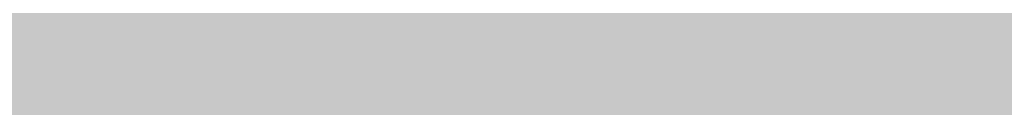
# Model space of a CAD drawing. Units: inches. Extents: x 2091 to 2899, y 967 to 2217.
# Tile 230 of 256: x 2203.4104 to 2203.7172, y 1152.274 to 1152.3009. Entities that reach past the tile are written whole.
import ezdxf

# ---------------------------------------------------------------- set-up
doc = ezdxf.new("R2010")
doc.units = ezdxf.units.IN
doc.layers.add('A-WALL-PATT', color=141, linetype='Continuous', lineweight=13, true_color=0xadddf7)

msp = doc.modelspace()

# ---------------------------------------------------------------- hatches: boundary and pattern name
at = {"layer": 'A-WALL-PATT'}
h = msp.add_hatch(color=256, dxfattribs=at)
h.dxf.hatch_style = 1
h.paths.add_polyline_path([(2803.1436, 2050.91906), (2203.1436, 2050.91906), (2203.1436, 1090.91906), (2803.1436, 1090.91906)])
h.paths.add_polyline_path([(2635.79885, 1147.54046), (2674.52405, 1147.54046, 0.376086), (2678.52967, 1152.8802), (2678.52967, 1159.55647, 0.333335), (2674.52432, 1163.56185), (2674.52432, 1163.56185), (2674.52432, 1192.93439), (2635.80597, 1192.93439), (2597.08762, 1192.93439), (2597.08762, 1163.56185, 0.333335), (2593.08228, 1159.55647), (2593.08228, 1152.8802, 0.376086), (2597.08789, 1147.54046)], flags=0)
h.paths.add_polyline_path([(2436.01043, 1278.24078, 0.000483), (2435.95264, 1278.21503, -0.001328), (2435.93563, 1278.11169, -0.001711), (2436.11644, 1278.04076, 0.002185)], flags=0)
h.paths.add_polyline_path([(2794.1436, 1143.41906), (2794.1436, 1347.41906), (2543.37017, 1347.41906), (2543.37017, 1351.91906), (2794.1436, 1351.91906), (2794.1436, 1392.71355), (2793.9474, 1392.71355), (2793.9474, 1473.5369), (2794.1436, 1473.5369), (2794.1436, 1531.91906), (2650.1436, 1531.91906), (2650.1436, 1536.41906), (2794.1436, 1536.41906), (2794.1436, 1692.41906), (2609.37561, 1692.41906), (2609.37561, 1644.41906), (2604.87561, 1644.41906), (2604.87561, 1744.91906), (2609.37561, 1744.91906), (2609.37561, 1696.91906), (2794.1436, 1696.91906), (2794.1436, 1780.91906), (2609.6436, 1780.91906), (2493.87561, 1780.91906), (2493.87561, 1785.41906), (2609.6436, 1785.41906), (2794.1436, 1785.41906), (2794.1436, 1847.93882), (2793.95122, 1847.93882), (2793.95122, 1928.76217), (2794.1436, 1928.76217), (2794.1436, 1941.41906), (2614.1436, 1941.41906), (2614.1436, 1821.41906), (2609.6436, 1821.41906), (2609.6436, 1941.41906), (2392.1436, 1941.41906), (2392.1436, 1819.91906), (2387.6436, 1819.91906), (2387.6436, 1941.41906), (2212.1436, 1941.41906), (2212.1436, 1783.91906), (2392.1436, 1783.91906), (2392.1436, 1780.91906), (2212.1436, 1780.91906), (2212.1436, 1629.41906), (2387.6436, 1629.41906), (2387.6436, 1744.91906), (2392.1436, 1744.91906), (2392.1436, 1627.91906), (2317.1436, 1627.91906), (2317.1436, 1551.41906), (2317.1436, 1536.41906), (2459.38359, 1536.41906), (2459.38359, 1602.39648), (2463.88359, 1602.39648), (2463.88359, 1531.91906), (2456.6436, 1531.91906), (2456.6436, 1529.91906), (2452.1436, 1529.91906), (2452.1436, 1531.91906), (2312.6436, 1531.91906), (2312.6436, 1551.41906), (2306.1436, 1551.41906), (2306.1436, 1555.91906), (2308.1436, 1555.91906), (2308.1436, 1551.41906), (2312.6436, 1551.41906), (2312.6436, 1627.91906), (2212.1436, 1627.91906), (2212.1436, 1555.91906), (2270.1436, 1555.91906), (2270.1436, 1551.41906), (2212.1436, 1551.41906), (2212.1436, 1351.91906), (2272.1436, 1351.91906), (2272.1436, 1347.41906), (2212.1436, 1347.41906), (2212.1436, 1275.41906), (2308.1436, 1275.41906), (2308.1436, 1351.91906), (2452.1436, 1351.91906), (2452.1436, 1493.91906), (2456.6436, 1493.91906), (2456.6436, 1347.41906), (2312.6436, 1347.41906), (2312.6436, 1270.91906), (2212.1436, 1270.91906), (2212.1436, 1099.91906), (2281.23752, 1099.91906), (2282.87104, 1110.9138), (2282.00834, 1116.9966), (2278.55774, 1121.4204), (2268.20564, 1128.0562), (2272.08764, 1128.0562), (2273.81294, 1131.927), (2279.42034, 1134.6919), (2285.02784, 1135.2449), (2287.61584, 1137.4568), (2288.04714, 1138.0098), (2289.34114, 1140.7747), (2291.06654, 1139.6687), (2292.36054, 1135.2449), (2295.37984, 1136.9038), (2296.24254, 1135.7979), (2297.10524, 1133.033), (2300.12464, 1138.0098), (2303.14394, 1138.0098), (2304.43794, 1135.7979), (2303.14394, 1133.586), (2306.59464, 1134.6919), (2307.88874, 1133.033), (2310.90804, 1135.2449), (2313.92744, 1134.1389), (2315.62686, 1132.4271), (2308.32004, 1117.5496), (2290.20384, 1109.8079), (2288.90984, 1103.1721), (2289.27231, 1099.91906), (2434.91823, 1099.91906), (2431.59323, 1124.78806), (2429.93023, 1169.55306), (2430.92718, 1240.51969), (2435.65893, 1238.18613), (2437.13523, 1196.55406), (2438.79823, 1143.97306), (2442.67823, 1111.99806), (2446.55823, 1099.91906), (2794.1436, 1099.91906), (2794.1436, 1138.91906), (2548.03245, 1138.91906), (2548.03245, 1143.41906), (2548.03245, 1148.81906), (2546.66846, 1148.03156), (2528.68569, 1179.17862, 0.256256), (2512.03245, 1148.81906), (2512.03245, 1143.41906), (2512.03245, 1138.91906), (2507.53245, 1138.91906), (2507.53245, 1143.41906), (2507.53245, 1148.81906, 0.256256), (2490.8792, 1179.17862), (2472.89644, 1148.03156), (2471.53245, 1148.81906), (2471.53245, 1143.41906), (2467.03245, 1143.41906), (2467.03245, 1269.94579, 0.039061), (2460.90999, 1273.58006), (2467.03245, 1273.58006), (2467.03245, 1286.32536, 0.014511), (2465.21619, 1286.76191), (2467.03245, 1287.05258), (2467.03245, 1323.41906), (2471.53245, 1323.41906), (2471.53245, 1148.81906), (2489.53245, 1179.99597), (2490.89644, 1179.20847), (2490.8792, 1179.17862, -0.256256), (2507.53245, 1148.81906), (2507.53245, 1143.41906), (2512.03245, 1143.41906), (2512.03245, 1148.81906, -0.256256), (2528.68569, 1179.17862), (2528.66846, 1179.20847), (2530.03245, 1179.99597), (2548.03245, 1148.81906), (2548.03245, 1143.41906)], flags=16)
h.paths.add_polyline_path([(2607.76855, 1200.94508), (2607.76855, 1265.03063), (2597.08762, 1281.05201), (2619.78459, 1281.05201), (2627.79528, 1337.12686), (2635.79885, 1337.12686), (2643.81666, 1337.12686), (2651.82736, 1281.05201), (2674.52432, 1281.05201), (2663.8434, 1265.03063), (2663.8434, 1200.94508), (2635.80597, 1200.94508)], flags=0)
edge = h.paths.add_edge_path(flags=0)
edge.add_ellipse((13303.89622, 1272.99872), major_axis=(-10595.31304, 0), ratio=0.84230387009, start_angle=0.628237219, end_angle=0.6465541, ccw=False)
edge.add_ellipse((2711.70045, 1156.85268), major_axis=(2.21977, 0), ratio=0.8423039, start_angle=111.53524, end_angle=180.62824, ccw=False)
edge.add_ellipse((13303.15629, 1272.99872), major_axis=(-10593.02631, 0), ratio=0.84230386954, start_angle=0.528271472, end_angle=0.646554097, ccw=False)
edge.add_line((2710.7646, 1175.3333), (2710.12999, 1175.3333))
edge.add_ellipse((2710.12999, 1176.57978), major_axis=(1.47985, 0), ratio=0.8423039, start_angle=180, end_angle=270, ccw=False)
edge.add_line((2708.65014, 1176.57978), (2708.65014, 1200.78291))
edge.add_ellipse((2710.12999, 1200.78291), major_axis=(1.47985, 0), ratio=0.8423039, start_angle=90, end_angle=180, ccw=False)
edge.add_line((2710.12999, 1202.02939), (2710.46508, 1202.02939))
edge.add_ellipse((13303.15629, 1272.99872), major_axis=(-10593.02631, 0), ratio=0.84230386954, start_angle=-0.090229089, end_angle=0.383866779, ccw=False)
edge.add_ellipse((2710.12999, 1290.92703), major_axis=(-1.47985, 0), ratio=0.8423039, start_angle=0, end_angle=90, ccw=False)
edge.add_line((2708.65014, 1290.92703), (2708.65014, 1315.13017))
edge.add_ellipse((2710.12999, 1315.13017), major_axis=(-1.47985, 0), ratio=0.8423039, start_angle=-90, end_angle=0, ccw=False)
edge.add_line((2710.12999, 1316.37665), (2710.70631, 1316.37665))
edge.add_ellipse((3238.40172, 1296.28957), major_axis=(528.234, 0), ratio=0.84230387, start_angle=176.3495724, end_angle=177.8200497, ccw=False)
edge.add_ellipse((2775.06304, 1071.4507), major_axis=(313.30776, 0), ratio=0.84230387, start_angle=102.1259656, end_angle=103.780529, ccw=False)
edge.add_ellipse((2775.06304, 1078.3057), major_axis=(-305.30289, 0), ratio=0.84230387, start_angle=-79.790461, end_angle=-77.5553727, ccw=False)
edge.add_ellipse((2695.14177, 1541.97538), major_axis=(-250.96022, 0), ratio=0.84230387, start_angle=99.256566, end_angle=102.5549326)
edge.add_line((2741.41033, 1334.21426), (2747.13255, 1337.37848))
edge.add_ellipse((2747.53862, 1336.85748), major_axis=(-0.73992, 0), ratio=0.842304, start_angle=270, end_angle=307.93313, ccw=False)
edge.add_ellipse((2747.53862, 1336.85748), major_axis=(-0.73992, 0), ratio=0.842304, start_angle=232.06687, end_angle=270, ccw=False)
edge.add_line((2747.94469, 1337.37848), (2753.66691, 1334.21426))
edge.add_ellipse((2799.93547, 1541.97538), major_axis=(250.96022, 0), ratio=0.84230387, start_angle=257.4450674, end_angle=260.743434)
edge.add_ellipse((2720.01419, 1078.3057), major_axis=(305.30289, 0), ratio=0.84230387, start_angle=77.5553727, end_angle=79.790461, ccw=False)
edge.add_ellipse((2720.01419, 1071.4507), major_axis=(-313.30776, 0), ratio=0.84230387, start_angle=256.219471, end_angle=257.8740344, ccw=False)
edge.add_ellipse((2256.67551, 1296.28957), major_axis=(-528.234, 0), ratio=0.84230387, start_angle=182.1799503, end_angle=183.6504276, ccw=False)
edge.add_line((2784.37092, 1316.37665), (2784.94725, 1316.37665))
edge.add_ellipse((2784.94725, 1315.13017), major_axis=(1.47985, 0), ratio=0.8423039, start_angle=0, end_angle=90, ccw=False)
edge.add_line((2786.42709, 1315.13017), (2786.42709, 1290.92703))
edge.add_ellipse((2784.94725, 1290.92703), major_axis=(1.47985, 0), ratio=0.8423039, start_angle=270, end_angle=360, ccw=False)
edge.add_ellipse((-7808.07906, 1272.99872), major_axis=(10593.02631, 0), ratio=0.84230386954, start_angle=-0.383866779, end_angle=0.090229089, ccw=False)
edge.add_line((2784.61216, 1202.02939), (2784.94725, 1202.02939))
edge.add_ellipse((2784.94725, 1200.78291), major_axis=(1.47985, 0), ratio=0.8423039, start_angle=0, end_angle=90, ccw=False)
edge.add_line((2786.42709, 1200.78291), (2786.42709, 1176.57978))
edge.add_ellipse((2784.94725, 1176.57978), major_axis=(-1.47985, 0), ratio=0.8423039, start_angle=90, end_angle=180, ccw=False)
edge.add_line((2784.94725, 1175.3333), (2784.31264, 1175.3333))
edge.add_ellipse((-7808.07906, 1272.99872), major_axis=(10593.02631, 0), ratio=0.84230386954, start_angle=-0.618643196, end_angle=-0.528271472, ccw=False)
edge.add_ellipse((2783.37678, 1156.85268), major_axis=(-2.21977, 0), ratio=0.8423039, start_angle=179.37176, end_angle=248.46476, ccw=False)
edge.add_ellipse((-7808.81898, 1272.99872), major_axis=(-10595.31304, 0), ratio=0.84230386576, start_angle=179.353445923, end_angle=179.371762803, ccw=False)
edge.add_ellipse((2780.2973, 1153.50079), major_axis=(-5.24643, 0), ratio=0.8423039, start_angle=90, end_angle=179.35345, ccw=False)
edge.add_line((2780.2973, 1149.08171), (2714.77993, 1149.08171))
edge.add_ellipse((2714.77993, 1153.50079), major_axis=(5.24643, 0), ratio=0.8423039, start_angle=180.64655, end_angle=270, ccw=False)
edge = h.paths.add_edge_path(flags=0)
edge.add_line((2718.18737, 1151.00783), (2718.18737, 1170.47236))
edge.add_ellipse((2721.14706, 1170.47236), major_axis=(-2.95969, 0), ratio=0.8423039, start_angle=-90, end_angle=0, ccw=False)
edge.add_line((2721.14706, 1172.96532), (2773.93017, 1172.96532))
edge.add_ellipse((2773.93017, 1170.47236), major_axis=(-2.95969, 0), ratio=0.8423039, start_angle=180, end_angle=270, ccw=False)
edge.add_line((2776.88987, 1170.47236), (2776.88987, 1151.00783))
edge.add_line((2776.88987, 1151.00783), (2718.18737, 1151.00783))
edge = h.paths.add_edge_path(flags=0)
edge.add_line((2718.18737, 1180.23415), (2718.18737, 1199.05783))
edge.add_ellipse((2747.53862, 1320.39864), major_axis=(147.01792, 0), ratio=0.84230387, start_angle=256.4018653, end_angle=283.5981347)
edge.add_line((2776.88987, 1199.05783), (2776.88987, 1180.23415))
edge.add_ellipse((2747.53862, 1301.57496), major_axis=(147.01792, 0), ratio=0.84230387, start_angle=256.4018653, end_angle=283.5981347, ccw=False)
edge = h.paths.add_edge_path(flags=0)
edge.add_ellipse((13303.15629, 1272.99872), major_axis=(-10591.54646, 0), ratio=0.84230386955, start_angle=0.055594314, end_angle=0.377764194, ccw=False)
edge.add_line((2711.61686, 1262.72171), (2715.66741, 1249.4954))
edge.add_ellipse((6413.89196, 1241.69192), major_axis=(-3698.23616, 0), ratio=0.8423038695, start_angle=-0.12089737, end_angle=0.36407635)
edge.add_line((2715.76104, 1218.19245), (2711.93431, 1203.16736))
edge = h.paths.add_edge_path(flags=0)
edge.add_line((2718.18737, 1251.07457), (2716.00249, 1267.45044))
edge.add_ellipse((2742.15117, 1202.18954), major_axis=(81.77258, 0), ratio=0.84230387, start_angle=94.277421, end_angle=111.8349538, ccw=False)
edge.add_line((2737.00975, 1270.93063), (2758.06748, 1270.93063))
edge.add_ellipse((2752.92606, 1202.18954), major_axis=(81.77258, 0), ratio=0.84230387, start_angle=68.1650462, end_angle=85.722579, ccw=False)
edge.add_line((2779.07475, 1267.45044), (2776.88987, 1251.07457))
edge.add_ellipse((2750.33806, 1187.88536), major_axis=(79.57966, 0), ratio=0.84230387, start_angle=67.2080851, end_angle=85.1299304)
edge.add_line((2756.03466, 1254.74366), (2739.04258, 1254.74366))
edge.add_ellipse((2744.73917, 1187.88536), major_axis=(79.57966, 0), ratio=0.84230387, start_angle=94.8700696, end_angle=112.7919149)
edge = h.paths.add_edge_path(flags=0)
edge.add_line((2783.14293, 1203.16736), (2779.31619, 1218.19245))
edge.add_ellipse((-918.81473, 1241.69192), major_axis=(3698.23616, 0), ratio=0.8423038695, start_angle=-0.36407635, end_angle=0.12089737)
edge.add_line((2779.40983, 1249.4954), (2783.46037, 1262.72171))
edge.add_ellipse((-7808.07906, 1272.99872), major_axis=(-10591.54646, 0), ratio=0.84230386954, start_angle=179.622235806, end_angle=179.944405687, ccw=False)
edge = h.paths.add_edge_path(flags=0)
edge.add_ellipse((2734.20089, 1286.69044), major_axis=(-0.35661, 6.34008), ratio=0.6038336, start_angle=89.002014, end_angle=253.657408, ccw=False)
edge.add_line((2730.369, 1286.54181), (2730.369, 1301.35198))
edge.add_line((2730.369, 1301.35198), (2735.91331, 1305.2148))
edge.add_ellipse((2736.38492, 1304.73456), major_axis=(0.73992, 0), ratio=0.842304, start_angle=90, end_angle=134.48021, ccw=False)
edge.add_line((2736.38492, 1305.3578), (2738.03278, 1305.3578))
edge.add_line((2738.03278, 1305.3578), (2738.03278, 1307.70793))
edge.add_ellipse((2794.20164, 1307.70793), major_axis=(56.16886, 0), ratio=0.84230387, start_angle=150.56143, end_angle=180, ccw=False)
edge.add_ellipse((2700.87559, 1307.70793), major_axis=(-56.16886, 0), ratio=0.84230387, start_angle=180, end_angle=209.43857, ccw=False)
edge.add_line((2757.04445, 1307.70793), (2757.04445, 1305.3578))
edge.add_line((2757.04445, 1305.3578), (2758.69232, 1305.3578))
edge.add_ellipse((2758.69232, 1304.73456), major_axis=(-0.73992, 0), ratio=0.842304, start_angle=225.51979, end_angle=270, ccw=False)
edge.add_line((2759.16392, 1305.2148), (2764.70823, 1301.35198))
edge.add_line((2764.70823, 1301.35198), (2764.70823, 1286.54181))
edge.add_ellipse((2760.87634, 1286.69044), major_axis=(0.35661, 6.34008), ratio=0.6038336, start_angle=106.342592, end_angle=270.997986, ccw=False)
edge.add_line((2757.04445, 1285.79709), (2757.04445, 1307.70793))
edge.add_ellipse((2700.87559, 1307.70793), major_axis=(-56.16886, 0), ratio=0.84230387, start_angle=180, end_angle=209.43857)
edge.add_ellipse((2794.20164, 1307.70793), major_axis=(56.16886, 0), ratio=0.84230387, start_angle=150.56143, end_angle=180)
edge.add_line((2738.03278, 1307.70793), (2738.03278, 1285.79709))
h.paths.add_polyline_path([(2417.81227, 1104.4497), (2413.49227, 1102.5297), (2410.61227, 1103.9697), (2409.17227, 1106.3697), (2407.25227, 1107.3297), (2406.29227, 1109.7297), (2405.33227, 1114.0497), (2405.33227, 1117.8897), (2406.29227, 1120.1297), (2407.25227, 1119.8097), (2408.84832, 1118.32766), (2410.17395, 1119.42417), (2410.21127, 1120.4057), (2411.04073, 1121.41905), (2410.69927, 1119.8587), (2410.17395, 1119.42417), (2410.08845, 1117.17611), (2411.13284, 1116.20632), (2413.97227, 1119.3297), (2416.85227, 1120.7697), (2416.86972, 1120.79878), (2417.03507, 1119.40512), (2417.89621, 1118.14338), (2418.29227, 1118.3697), (2419.54445, 1120.03927), (2419.36092, 1118.38749), (2419.03211, 1119.35615), (2418.39894, 1118.51193), (2419.25227, 1114.5297), (2418.79409, 1107.19879)], flags=0)
h.paths.add_polyline_path([(2508.87017, 1347.41906), (2508.37017, 1347.41906), (2508.37017, 1351.91906), (2508.87017, 1351.91906)], flags=0)
h.paths.add_polyline_path([(2473.37017, 1347.41906), (2472.37017, 1347.41906), (2467.87017, 1347.41906), (2467.87017, 1455.41906), (2472.37017, 1455.41906), (2472.37017, 1352.41906), (2473.37017, 1352.41906)], flags=0)
h.paths.add_polyline_path([(2352.10624, 1217.4462), (2349.22624, 1218.8862), (2347.78624, 1221.2862), (2345.86624, 1222.2462), (2344.90624, 1224.6462), (2343.94624, 1228.9662), (2343.94624, 1232.8062), (2344.90624, 1235.0462), (2345.86624, 1234.7262), (2347.46229, 1233.24415), (2348.78792, 1234.34066), (2348.82524, 1235.3222), (2349.6547, 1236.33555), (2349.31324, 1234.7752), (2348.78792, 1234.34066), (2348.70242, 1232.0926), (2349.74681, 1231.12282), (2352.58624, 1234.2462), (2355.46624, 1235.6862), (2355.48369, 1235.71528), (2355.64904, 1234.32161), (2356.51018, 1233.05988), (2356.90624, 1233.2862), (2358.15842, 1234.95576), (2357.97489, 1233.30398), (2357.64608, 1234.27264), (2357.01291, 1233.42842), (2357.86624, 1229.4462), (2357.40806, 1222.11529), (2356.42624, 1219.3662)], flags=0)
h.paths.add_polyline_path([(2348.2968, 1112.22442), (2347.0138, 1112.31042), (2345.5298, 1114.12742), (2345.7318, 1115.85842), (2346.8118, 1116.98242), (2346.8118, 1114.64642), (2345.8668, 1114.21442), (2346.8798, 1114.30042)], flags=0)
h.paths.add_polyline_path([(2347.0138, 1110.92642), (2346.2718, 1110.49342), (2346.6098, 1111.18642)], flags=0)
h.paths.add_polyline_path([(2345.8668, 1118.19442), (2345.5298, 1117.32942), (2343.7078, 1118.02142), (2344.3828, 1118.62642)], flags=0)
h.paths.add_polyline_path([(2346.6768, 1109.28242), (2346.0698, 1108.07142), (2345.8668, 1110.06142)], flags=0)
h.paths.add_polyline_path([(2345.0568, 1119.75142), (2343.6398, 1119.75142), (2343.9778, 1121.13542)], flags=0)
h.paths.add_polyline_path([(2345.2598, 1116.55042), (2345.1248, 1115.85842), (2344.9218, 1115.68542), (2344.7198, 1116.37742)], flags=0)
h.paths.add_polyline_path([(2345.6648, 1112.31042), (2345.4618, 1111.53242), (2344.0448, 1111.96442), (2344.6518, 1112.57042)], flags=0)
h.paths.add_polyline_path([(2345.1918, 1113.34942), (2344.4498, 1113.86842), (2344.7198, 1114.38742)], flags=0)
h.paths.add_polyline_path([(2344.6518, 1116.80942), (2344.1798, 1115.68542), (2344.6518, 1115.33942), (2343.9098, 1114.90642), (2343.0328, 1115.94442), (2343.6398, 1116.46342)], flags=0)
h.paths.add_polyline_path([(2345.8668, 1106.68642), (2344.9898, 1105.56242), (2344.5168, 1106.60042)], flags=0)
h.paths.add_polyline_path([(2344.8548, 1110.06142), (2344.5168, 1109.28242), (2344.1128, 1109.71542)], flags=0)
h.paths.add_polyline_path([(2344.0448, 1113.52242), (2343.4378, 1113.08942), (2342.7628, 1113.95442)], flags=0)
h.paths.add_polyline_path([(2344.3148, 1111.01242), (2342.9648, 1110.32042), (2342.9648, 1111.09942)], flags=0)
h.paths.add_polyline_path([(2345.1248, 1104.69742), (2344.5848, 1103.74542), (2344.4498, 1104.26442)], flags=0)
h.paths.add_polyline_path([(2342.8298, 1121.22242), (2341.7498, 1120.53042), (2340.5358, 1121.04942), (2340.1308, 1121.82842), (2340.6708, 1122.95242), (2341.1428, 1121.82842), (2341.6148, 1122.00142)], flags=0)
h.paths.add_polyline_path([(2342.9648, 1119.75142), (2343.0328, 1118.45342), (2342.0878, 1118.02142), (2342.0198, 1119.49142)], flags=0)
h.paths.add_polyline_path([(2342.6948, 1116.89642), (2341.9528, 1116.63642), (2342.0198, 1117.32942)], flags=0)
h.paths.add_polyline_path([(2343.0328, 1112.22442), (2342.0198, 1111.79142), (2341.5478, 1112.22442), (2342.3578, 1113.34942)], flags=0)
h.paths.add_polyline_path([(2343.7748, 1104.43742), (2342.6278, 1102.88042), (2342.6948, 1104.61042), (2343.4378, 1105.12942)], flags=0)
h.paths.add_polyline_path([(2342.0198, 1115.07942), (2340.8058, 1115.51242), (2340.9408, 1116.37742)], flags=0)
h.paths.add_polyline_path([(2341.4808, 1120.09742), (2341.4808, 1119.40542), (2341.0758, 1119.57842), (2341.1428, 1120.09742)], flags=0)
h.paths.add_polyline_path([(2341.8178, 1114.47342), (2340.9408, 1113.08942), (2340.8058, 1114.56042)], flags=0)
h.paths.add_polyline_path([(2341.1428, 1118.54042), (2340.9408, 1116.98242), (2339.0508, 1117.67542), (2339.0508, 1118.62642)], flags=0)
h.paths.add_polyline_path([(2342.6948, 1101.66842), (2341.9528, 1101.84142), (2342.5598, 1102.36142)], flags=0)
h.paths.add_polyline_path([(2340.3328, 1119.66542), (2338.4438, 1119.57842), (2337.9038, 1120.35742), (2339.6578, 1120.61642)], flags=0)
h.paths.add_polyline_path([(2340.3328, 1115.33942), (2340.0628, 1113.69542), (2339.3878, 1115.33942)], flags=0)
h.paths.add_polyline_path([(2341.8178, 1103.83142), (2341.5478, 1102.88042), (2341.1428, 1103.65842)], flags=0)
h.paths.add_polyline_path([(2339.0508, 1122.86642), (2337.2958, 1121.82842), (2337.0938, 1123.12542), (2337.7688, 1123.81842)], flags=0)
h.paths.add_polyline_path([(2339.1178, 1121.74142), (2338.8478, 1121.22242), (2338.1738, 1121.04942), (2338.3758, 1121.56842)], flags=0)
h.paths.add_polyline_path([(2339.1858, 1119.31942), (2338.6458, 1118.71342), (2338.2408, 1118.10742), (2338.2408, 1118.88642)], flags=0)
h.paths.add_polyline_path([(2341.1428, 1101.92842), (2340.6028, 1101.23642), (2340.0628, 1101.84142), (2340.6028, 1102.36142)], flags=0)
h.paths.add_polyline_path([(2337.6338, 1117.76142), (2336.6208, 1118.28042), (2337.2958, 1118.97242)], flags=0)
h.paths.add_polyline_path([(2336.8238, 1119.57842), (2334.7988, 1118.97242), (2335.2038, 1120.35742), (2336.5538, 1120.87642)], flags=0)
h.paths.add_polyline_path([(2339.1178, 1100.45742), (2337.3638, 1100.54342), (2336.7558, 1101.23642)], flags=0)
h.paths.add_polyline_path([(2336.3508, 1122.43342), (2336.0138, 1121.91442), (2334.9338, 1122.43342), (2334.5288, 1123.47142), (2335.7438, 1122.77942)], flags=0)
h.paths.add_polyline_path([(2334.7318, 1120.87642), (2334.2588, 1120.35742), (2334.0568, 1120.78942), (2334.5968, 1121.30842)], flags=0)
h.paths.add_polyline_path([(2334.4618, 1122.17442), (2332.5718, 1121.30842), (2331.3568, 1122.17442), (2332.0998, 1122.86642)], flags=0)
h.paths.add_polyline_path([(2334.2588, 1118.54042), (2333.3818, 1118.45342), (2333.6518, 1119.31942)], flags=0)
h.paths.add_polyline_path([(2335.5418, 1102.27442), (2334.1918, 1102.62042), (2335.2718, 1103.31242)], flags=0)
h.paths.add_polyline_path([(2332.7068, 1119.66542), (2331.6948, 1120.44342), (2332.5048, 1120.78942)], flags=0)
h.paths.add_polyline_path([(2334.7318, 1101.14942), (2333.5168, 1101.58242), (2333.9888, 1101.75542)], flags=0)
h.paths.add_polyline_path([(2332.6398, 1116.63642), (2331.0868, 1116.29042), (2331.9648, 1118.19442)], flags=0)
h.paths.add_polyline_path([(2330.7498, 1121.56842), (2330.2768, 1120.27042), (2328.5228, 1119.31942), (2328.9948, 1121.04942)], flags=0)
h.paths.add_polyline_path([(2330.7498, 1118.62642), (2330.0078, 1117.50242), (2329.8728, 1118.02142)], flags=0)
h.paths.add_polyline_path([(2332.0998, 1102.36142), (2330.5468, 1102.01442), (2331.6948, 1102.96642)], flags=0)
h.paths.add_polyline_path([(2329.5348, 1113.60842), (2329.0628, 1112.31042), (2328.5898, 1113.34942)], flags=0)
h.paths.add_polyline_path([(2328.3878, 1117.84842), (2327.5098, 1116.55042), (2327.1728, 1117.76142)], flags=0)
h.paths.add_polyline_path([(2329.7378, 1106.51342), (2329.5348, 1105.30242), (2328.2528, 1106.08142)], flags=0)
h.paths.add_polyline_path([(2328.6578, 1114.38742), (2328.0498, 1114.12742), (2328.3198, 1114.90642)], flags=0)
h.paths.add_polyline_path([(2328.3198, 1112.22442), (2327.1058, 1112.13742), (2326.7008, 1112.65642)], flags=0)
h.paths.add_polyline_path([(2326.9028, 1115.25242), (2326.7008, 1114.12742), (2325.2158, 1113.60842), (2326.0928, 1115.33942)], flags=0)
h.paths.add_polyline_path([(2326.6328, 1108.33042), (2326.0928, 1107.37942), (2325.8908, 1108.50342), (2326.4978, 1109.10942)], flags=0)
h.paths.add_polyline_path([(2615.1436, 1531.91906), (2609.6436, 1531.91906), (2609.6436, 1620.41906), (2614.1436, 1620.41906), (2614.1436, 1536.41906), (2615.1436, 1536.41906)], flags=0)
h.paths.add_polyline_path([(2545.1436, 1563.41906), (2464.1436, 1563.41906), (2464.1436, 1632.41906), (2509.1436, 1632.41906), (2509.1436, 1627.91906), (2509.1436, 1603.91906), (2468.6436, 1603.91906), (2468.6436, 1567.91906), (2540.6436, 1567.91906), (2540.6436, 1591.91906), (2545.1436, 1591.91906)], flags=0)
h.paths.add_polyline_path([(2388.96905, 1549.98573), (2357.43418, 1549.98573), (2357.43418, 1623.36078), (2399.36278, 1623.36078), (2435.68947, 1623.36078), (2435.59255, 1602.55927), (2435.59255, 1602.39648), (2388.96905, 1602.39648)], flags=0)
h.paths.add_polyline_path([(2388.88063, 1555.80915), (2374.90443, 1555.80915), (2374.90443, 1600.57156), (2374.90443, 1615.45765), (2406.35088, 1615.45765), (2406.35088, 1618.93943), (2412.17429, 1615.45765), (2406.35088, 1611.97586), (2406.35088, 1615.45765), (2388.88063, 1615.45765)], flags=0)
h.paths.add_polyline_path([(2568.87561, 1644.41906), (2453.37561, 1644.41906), (2453.37561, 1785.41906), (2457.87561, 1785.41906), (2457.87561, 1648.91906), (2568.87561, 1648.91906)], flags=0)
h.paths.add_polyline_path([(2212.1436, 1945.91906), (2212.1436, 2041.91906), (2794.1436, 2041.91906), (2794.1436, 1945.91906)], flags=16)
h.paths.add_polyline_path([(2271.08273, 1964.31724), (2776.85297, 1964.31724), (2776.85297, 2037.16962), (2271.08273, 2037.16962)], flags=8)
h.paths.add_polyline_path([(2380.64929, 1536.82414), (2461.04081, 1536.82414), (2461.04081, 1554.65259), (2380.64929, 1554.65259)], flags=8)
h.paths.add_polyline_path([(2240.75571, 1609.72545), (2309.18583, 1609.72545), (2309.18583, 1617.6982), (2240.75571, 1617.6982)], flags=8)
h.paths.add_polyline_path([(2212.67726, 1313.5041), (2282.59152, 1313.5041), (2282.59152, 1322.74524), (2212.67726, 1322.74524)], flags=8)
h.paths.add_polyline_path([(2457.11198, 1114.77857), (2558.48158, 1114.77857), (2558.48158, 1142.21968), (2457.11198, 1142.21968)], flags=8)
h.paths.add_polyline_path([(2473.44234, 1273.01007), (2604.64123, 1273.01007), (2604.64123, 1318.34693), (2473.44234, 1318.34693)], flags=8)
h.paths.add_polyline_path([(2638.8763, 1626.97743), (2684.25037, 1627.97674), (2684.03848, 1637.59749), (2638.66442, 1636.59819)], flags=8)
h.paths.add_polyline_path([(2537.59055, 1453.79345), (2628.38955, 1453.79345), (2628.38955, 1475.34481), (2537.59055, 1475.34481)], flags=8)
h.paths.add_polyline_path([(2504.13764, 1714.6324), (2554.64719, 1714.6324), (2554.64719, 1730.23771), (2504.13764, 1730.23771)], flags=8)
h.paths.add_polyline_path([(2487.50118, 1575.65187), (2535.09712, 1575.65187), (2535.09712, 1598.37765), (2487.50118, 1598.37765)], flags=8)
h.paths.add_polyline_path([(2709.0994, 1735.71028), (2740.0166, 1735.71028), (2740.0166, 1749.93764), (2709.0994, 1749.93764)], flags=8)
h.paths.add_polyline_path([(2442.43842, 1792.17166), (2564.72884, 1792.17166), (2564.72884, 1842.00016), (2442.43842, 1842.00016)], flags=8)
h.paths.add_polyline_path([(2655.8158, 1809.64408), (2789.52014, 1806.6938), (2790.08498, 1832.29164), (2656.38064, 1835.24192)], flags=8)
h.paths.add_polyline_path([(2234.8427, 1797.72014), (2368.59285, 1794.76885), (2369.16072, 1820.50413), (2235.41056, 1823.45542)], flags=8)
h.paths.add_polyline_path([(2245.13847, 1644.00633), (2398.42773, 1640.6239), (2398.99484, 1666.32482), (2245.70557, 1669.70725)], flags=8)
h.paths.add_polyline_path([(2306.14285, 1431.16852), (2413.76831, 1428.79369), (2414.33315, 1454.39153), (2306.70768, 1456.76636)], flags=8)
h.paths.add_polyline_path([(2306.83458, 1458.23314), (2393.38048, 1456.32345), (2393.93281, 1481.35436), (2307.38691, 1483.26405)], flags=8)

doc.saveas('drawing.dxf')
